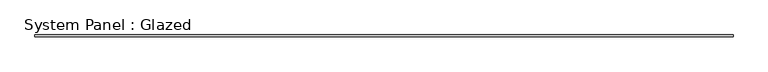
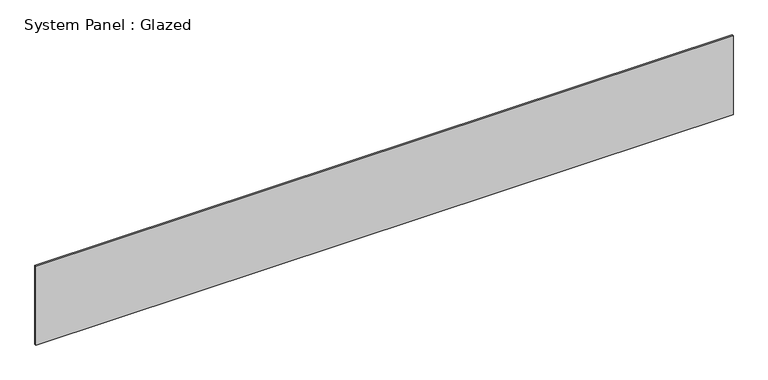
"""IFC4 building model written with IfcOpenShell, lengths in millimetres: plate geometry, System Panel : Glazed."""

from ifc_helpers import new_model, si_unit, origin, origin_with_axes, place, context, project, spatial, polyline, outline, extrude, source, transform, mapped, element, save


def system_panel_glazed_fdc1463f(model_context):
    return source(origin(), model_context, "Body", "SweptSolid", [
        extrude(outline(polyline([(5101.7485037, 19.05), (-5101.7485037, 19.05), (-5101.7485037, 44.45), (5101.7485037, 44.45), (5101.7485037, 19.05)])), origin_with_axes(), (0.0, 0.0, 1.0), 1219.2),
    ])


if __name__ == "__main__":
    model = new_model("IFC4")
    model_context = context("Model", 3, world=origin())
    ifc_project = project(units=[si_unit("LENGTHUNIT", "METRE", prefix="MILLI")], contexts=[model_context])
    site = spatial("IfcSite", under=ifc_project)
    building = spatial("IfcBuilding", under=site)
    placement = place(None, origin())
    system_panel_glazed_shape = system_panel_glazed_fdc1463f(model_context)
    element("IfcPlate", 1, ObjectType="System Panel : Glazed", at=placement, inside=building, context=model_context, shape_type="MappedRepresentation", body=[
        mapped(system_panel_glazed_shape, transform((0.0, 0.0, 0.0), x_axis=(1.0, 0.0, 0.0), y_axis=(0.0, 1.0, 0.0), z_axis=(0.0, 0.0, 1.0))),
    ])
    save(model, "model.ifc")

# Revit data of these elements
# Type "System Panel : Glazed"
#   Construction Type Id = "GSP4R"
#   Analytic Construction = "1/8 in Pilkington single glazing"
#   Visual Light Transmittance = 0.9
#   Solar Heat Gain Coefficient = 0.86
#   Heat Transfer Coefficient (U) = 1.18115 BTU/(h·ft²·°F)
# Element 1 (IfcPlate, "System Panel : Glazed")
#   Materials on its faces: "Glass"
# Materials
#   "Glass": class "Glass", colour RGB 0 128 192, transparency 0.75, Description = "Soda Lime Glass", Cost = 0
